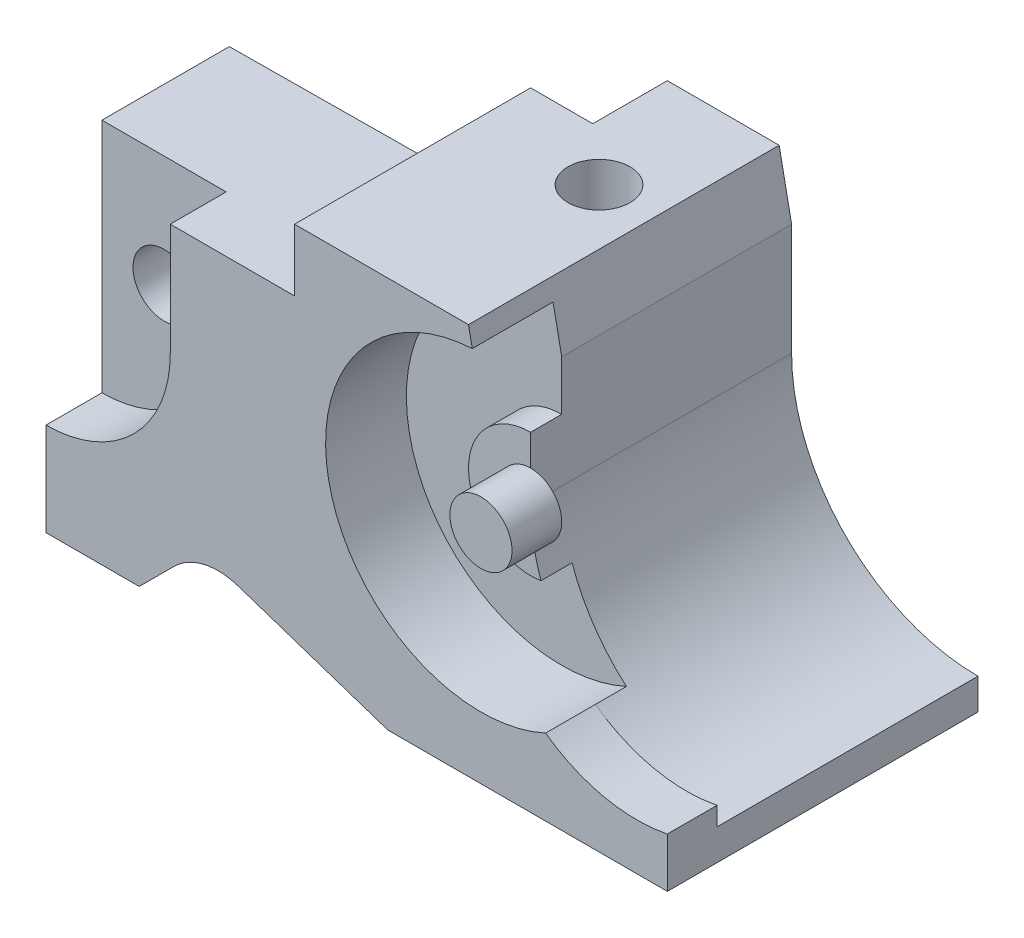
ISO-10303-21;
HEADER;
FILE_DESCRIPTION(('STEP AP214'),'2;1');
FILE_NAME('part.step','',(''),(''),'','','');
FILE_SCHEMA(('AUTOMOTIVE_DESIGN { 1 0 10303 214 1 1 1 1 }'));
ENDSEC;
DATA;
#1=APPLICATION_CONTEXT('core data for automotive mechanical design processes');
#2=APPLICATION_PROTOCOL_DEFINITION('international standard','automotive_design',2000,#1);
#3=PRODUCT_CONTEXT('',#1,'mechanical');
#4=PRODUCT('Part','Part','',(#3));
#5=PRODUCT_RELATED_PRODUCT_CATEGORY('part','',(#4));
#6=PRODUCT_DEFINITION_FORMATION('','',#4);
#7=PRODUCT_DEFINITION_CONTEXT('part definition',#1,'design');
#8=PRODUCT_DEFINITION('design','',#6,#7);
#9=PRODUCT_DEFINITION_SHAPE('','',#8);
#10=(LENGTH_UNIT() NAMED_UNIT(*) SI_UNIT(.MILLI.,.METRE.));
#11=(NAMED_UNIT(*) PLANE_ANGLE_UNIT() SI_UNIT($,.RADIAN.));
#12=(NAMED_UNIT(*) SI_UNIT($,.STERADIAN.) SOLID_ANGLE_UNIT());
#13=UNCERTAINTY_MEASURE_WITH_UNIT(LENGTH_MEASURE(1.E-05),#10,'distance_accuracy_value','');
#14=(GEOMETRIC_REPRESENTATION_CONTEXT(3) GLOBAL_UNCERTAINTY_ASSIGNED_CONTEXT((#13)) GLOBAL_UNIT_ASSIGNED_CONTEXT((#10,
#11,#12)) REPRESENTATION_CONTEXT('',''));
#15=CARTESIAN_POINT('',(0.,0.,0.));
#16=DIRECTION('',(0.,0.,1.));
#17=DIRECTION('',(1.,0.,0.));
#18=AXIS2_PLACEMENT_3D('',#15,#16,#17);
#19=CARTESIAN_POINT('',(0.,0.,50.));
#20=DIRECTION('',(0.,1.,0.));
#21=DIRECTION('',(0.,0.,1.));
#22=AXIS2_PLACEMENT_3D('',#19,#20,#21);
#23=PLANE('',#22);
#24=DIRECTION('',(-0.999964092712605,0.,0.00847427197214061));
#25=VECTOR('',#24,1.);
#26=CARTESIAN_POINT('',(0.173716337522439,0.,20.4985278276481));
#27=LINE('',#26,#25);
#28=CARTESIAN_POINT('',(15.,0.,20.3728813559322));
#29=VERTEX_POINT('',#28);
#30=CARTESIAN_POINT('',(0.,0.,20.5));
#31=VERTEX_POINT('',#30);
#32=EDGE_CURVE('E213',#29,#31,#27,.T.);
#33=ORIENTED_EDGE('',*,*,#32,.F.);
#34=DIRECTION('',(0.,0.,1.));
#35=VECTOR('',#34,1.);
#36=CARTESIAN_POINT('',(15.,0.,0.));
#37=LINE('',#36,#35);
#38=CARTESIAN_POINT('',(15.,0.,50.));
#39=VERTEX_POINT('',#38);
#40=EDGE_CURVE('E352',#29,#39,#37,.T.);
#41=ORIENTED_EDGE('',*,*,#40,.T.);
#42=DIRECTION('',(1.,0.,0.));
#43=VECTOR('',#42,1.);
#44=CARTESIAN_POINT('',(0.,0.,50.));
#45=LINE('',#44,#43);
#46=CARTESIAN_POINT('',(0.,0.,50.));
#47=VERTEX_POINT('',#46);
#48=EDGE_CURVE('E237',#47,#39,#45,.T.);
#49=ORIENTED_EDGE('',*,*,#48,.F.);
#50=DIRECTION('',(0.,0.,-1.));
#51=VECTOR('',#50,1.);
#52=CARTESIAN_POINT('',(0.,0.,50.));
#53=LINE('',#52,#51);
#54=EDGE_CURVE('E229',#47,#31,#53,.T.);
#55=ORIENTED_EDGE('',*,*,#54,.T.);
#56=EDGE_LOOP('',(#33,#41,#49,#55));
#57=FACE_BOUND('',#56,.T.);
#58=ADVANCED_FACE('F41',(#57),#23,.F.);
#59=CARTESIAN_POINT('',(0.,63.,50.));
#60=DIRECTION('',(0.,-1.,0.));
#61=DIRECTION('',(0.,0.,-1.));
#62=AXIS2_PLACEMENT_3D('',#59,#60,#61);
#63=PLANE('',#62);
#64=CARTESIAN_POINT('',(59.,63.,20.));
#65=DIRECTION('',(0.,1.,0.));
#66=DIRECTION('',(0.,0.,1.));
#67=AXIS2_PLACEMENT_3D('',#64,#65,#66);
#68=CIRCLE('',#67,5.);
#69=CARTESIAN_POINT('',(59.,63.,25.));
#70=VERTEX_POINT('',#69);
#71=EDGE_CURVE('E304',#70,#70,#68,.T.);
#72=ORIENTED_EDGE('',*,*,#71,.F.);
#73=EDGE_LOOP('',(#72));
#74=FACE_BOUND('',#73,.T.);
#75=DIRECTION('',(1.,0.,0.));
#76=VECTOR('',#75,1.);
#77=CARTESIAN_POINT('',(0.,63.,12.));
#78=LINE('',#77,#76);
#79=CARTESIAN_POINT('',(40.,63.,12.));
#80=VERTEX_POINT('',#79);
#81=CARTESIAN_POINT('',(50.,63.,12.));
#82=VERTEX_POINT('',#81);
#83=EDGE_CURVE('E303',#80,#82,#78,.T.);
#84=ORIENTED_EDGE('',*,*,#83,.F.);
#85=DIRECTION('',(0.,0.,-1.));
#86=VECTOR('',#85,1.);
#87=CARTESIAN_POINT('',(40.,63.,50.));
#88=LINE('',#87,#86);
#89=CARTESIAN_POINT('',(40.,63.,50.));
#90=VERTEX_POINT('',#89);
#91=EDGE_CURVE('E252',#90,#80,#88,.T.);
#92=ORIENTED_EDGE('',*,*,#91,.F.);
#93=DIRECTION('',(-1.,0.,0.));
#94=VECTOR('',#93,1.);
#95=CARTESIAN_POINT('',(0.,63.,50.));
#96=LINE('',#95,#94);
#97=CARTESIAN_POINT('',(68.,63.,50.));
#98=VERTEX_POINT('',#97);
#99=EDGE_CURVE('E423',#98,#90,#96,.T.);
#100=ORIENTED_EDGE('',*,*,#99,.F.);
#101=DIRECTION('',(0.,0.,-1.));
#102=VECTOR('',#101,1.);
#103=CARTESIAN_POINT('',(68.,63.,50.));
#104=LINE('',#103,#102);
#105=CARTESIAN_POINT('',(68.,63.,0.));
#106=VERTEX_POINT('',#105);
#107=EDGE_CURVE('E254',#98,#106,#104,.T.);
#108=ORIENTED_EDGE('',*,*,#107,.T.);
#109=DIRECTION('',(-1.,0.,0.));
#110=VECTOR('',#109,1.);
#111=CARTESIAN_POINT('',(0.,63.,0.));
#112=LINE('',#111,#110);
#113=CARTESIAN_POINT('',(50.,63.,0.));
#114=VERTEX_POINT('',#113);
#115=EDGE_CURVE('E445',#106,#114,#112,.T.);
#116=ORIENTED_EDGE('',*,*,#115,.T.);
#117=DIRECTION('',(0.,0.,-1.));
#118=VECTOR('',#117,1.);
#119=CARTESIAN_POINT('',(50.,63.,50.));
#120=LINE('',#119,#118);
#121=EDGE_CURVE('E301',#82,#114,#120,.T.);
#122=ORIENTED_EDGE('',*,*,#121,.F.);
#123=EDGE_LOOP('',(#84,#92,#100,#108,#116,#122));
#124=FACE_BOUND('',#123,.T.);
#125=ADVANCED_FACE('F494',(#74,#124),#63,.F.);
#126=CARTESIAN_POINT('',(40.,0.,50.));
#127=DIRECTION('',(1.,0.,0.));
#128=DIRECTION('',(0.,0.,-1.));
#129=AXIS2_PLACEMENT_3D('',#126,#127,#128);
#130=PLANE('',#129);
#131=ORIENTED_EDGE('',*,*,#91,.T.);
#132=DIRECTION('',(0.,1.,0.));
#133=VECTOR('',#132,1.);
#134=CARTESIAN_POINT('',(40.,0.,12.));
#135=LINE('',#134,#133);
#136=CARTESIAN_POINT('',(40.,5.,12.));
#137=VERTEX_POINT('',#136);
#138=EDGE_CURVE('E269',#137,#80,#135,.T.);
#139=ORIENTED_EDGE('',*,*,#138,.F.);
#140=DIRECTION('',(0.,0.,1.));
#141=VECTOR('',#140,1.);
#142=CARTESIAN_POINT('',(40.,5.,0.));
#143=LINE('',#142,#141);
#144=CARTESIAN_POINT('',(40.,4.99999999999999,20.1610169491525));
#145=VERTEX_POINT('',#144);
#146=EDGE_CURVE('E11',#137,#145,#143,.T.);
#147=ORIENTED_EDGE('',*,*,#146,.T.);
#148=DIRECTION('',(0.,1.,0.));
#149=VECTOR('',#148,1.);
#150=CARTESIAN_POINT('',(40.,0.,20.1610169491525));
#151=LINE('',#150,#149);
#152=CARTESIAN_POINT('',(40.,53.,20.1610169491525));
#153=VERTEX_POINT('',#152);
#154=EDGE_CURVE('E232',#145,#153,#151,.T.);
#155=ORIENTED_EDGE('',*,*,#154,.T.);
#156=DIRECTION('',(0.,0.,-1.));
#157=VECTOR('',#156,1.);
#158=CARTESIAN_POINT('',(40.,53.,50.));
#159=LINE('',#158,#157);
#160=CARTESIAN_POINT('',(40.,53.,50.));
#161=VERTEX_POINT('',#160);
#162=EDGE_CURVE('E245',#161,#153,#159,.T.);
#163=ORIENTED_EDGE('',*,*,#162,.F.);
#164=DIRECTION('',(0.,-1.,0.));
#165=VECTOR('',#164,1.);
#166=CARTESIAN_POINT('',(40.,0.,50.));
#167=LINE('',#166,#165);
#168=EDGE_CURVE('E425',#90,#161,#167,.T.);
#169=ORIENTED_EDGE('',*,*,#168,.F.);
#170=EDGE_LOOP('',(#131,#139,#147,#155,#163,#169));
#171=FACE_BOUND('',#170,.T.);
#172=ADVANCED_FACE('F286',(#171),#130,.F.);
#173=CARTESIAN_POINT('',(0.,53.,50.));
#174=DIRECTION('',(0.,-1.,0.));
#175=DIRECTION('',(0.,0.,-1.));
#176=AXIS2_PLACEMENT_3D('',#173,#174,#175);
#177=PLANE('',#176);
#178=DIRECTION('',(0.999964092712605,0.,-0.00847427197214061));
#179=VECTOR('',#178,1.);
#180=CARTESIAN_POINT('',(-0.249982046678632,53.,20.502118491921));
#181=LINE('',#180,#179);
#182=CARTESIAN_POINT('',(0.,53.,20.5));
#183=VERTEX_POINT('',#182);
#184=EDGE_CURVE('E287',#183,#153,#181,.T.);
#185=ORIENTED_EDGE('',*,*,#184,.F.);
#186=DIRECTION('',(0.,0.,-1.));
#187=VECTOR('',#186,1.);
#188=CARTESIAN_POINT('',(0.,53.,50.));
#189=LINE('',#188,#187);
#190=CARTESIAN_POINT('',(0.,53.,41.));
#191=VERTEX_POINT('',#190);
#192=EDGE_CURVE('E234',#191,#183,#189,.T.);
#193=ORIENTED_EDGE('',*,*,#192,.F.);
#194=DIRECTION('',(-1.,0.,0.));
#195=VECTOR('',#194,1.);
#196=CARTESIAN_POINT('',(0.,53.,41.));
#197=LINE('',#196,#195);
#198=CARTESIAN_POINT('',(20.,53.,41.));
#199=VERTEX_POINT('',#198);
#200=EDGE_CURVE('E325',#199,#191,#197,.T.);
#201=ORIENTED_EDGE('',*,*,#200,.F.);
#202=DIRECTION('',(0.,0.,1.));
#203=VECTOR('',#202,1.);
#204=CARTESIAN_POINT('',(20.,53.,41.));
#205=LINE('',#204,#203);
#206=CARTESIAN_POINT('',(20.,53.,50.));
#207=VERTEX_POINT('',#206);
#208=EDGE_CURVE('E328',#199,#207,#205,.T.);
#209=ORIENTED_EDGE('',*,*,#208,.T.);
#210=DIRECTION('',(-1.,0.,0.));
#211=VECTOR('',#210,1.);
#212=CARTESIAN_POINT('',(0.,53.,50.));
#213=LINE('',#212,#211);
#214=EDGE_CURVE('E428',#161,#207,#213,.T.);
#215=ORIENTED_EDGE('',*,*,#214,.F.);
#216=ORIENTED_EDGE('',*,*,#162,.T.);
#217=EDGE_LOOP('',(#185,#193,#201,#209,#215,#216));
#218=FACE_BOUND('',#217,.T.);
#219=ADVANCED_FACE('F538',(#218),#177,.F.);
#220=CARTESIAN_POINT('',(0.,0.,50.));
#221=DIRECTION('',(1.,0.,0.));
#222=DIRECTION('',(0.,0.,-1.));
#223=AXIS2_PLACEMENT_3D('',#220,#221,#222);
#224=PLANE('',#223);
#225=DIRECTION('',(0.,1.,0.));
#226=VECTOR('',#225,1.);
#227=CARTESIAN_POINT('',(0.,0.,20.5));
#228=LINE('',#227,#226);
#229=EDGE_CURVE('E217',#31,#183,#228,.T.);
#230=ORIENTED_EDGE('',*,*,#229,.F.);
#231=ORIENTED_EDGE('',*,*,#54,.F.);
#232=DIRECTION('',(0.,-1.,0.));
#233=VECTOR('',#232,1.);
#234=CARTESIAN_POINT('',(0.,0.,50.));
#235=LINE('',#234,#233);
#236=CARTESIAN_POINT('',(0.,15.,50.));
#237=VERTEX_POINT('',#236);
#238=EDGE_CURVE('E429',#237,#47,#235,.T.);
#239=ORIENTED_EDGE('',*,*,#238,.F.);
#240=DIRECTION('',(0.,0.,1.));
#241=VECTOR('',#240,1.);
#242=CARTESIAN_POINT('',(0.,15.,41.));
#243=LINE('',#242,#241);
#244=CARTESIAN_POINT('',(0.,15.,41.));
#245=VERTEX_POINT('',#244);
#246=EDGE_CURVE('E322',#245,#237,#243,.T.);
#247=ORIENTED_EDGE('',*,*,#246,.F.);
#248=DIRECTION('',(0.,-1.,0.));
#249=VECTOR('',#248,1.);
#250=CARTESIAN_POINT('',(0.,0.,41.));
#251=LINE('',#250,#249);
#252=EDGE_CURVE('E312',#191,#245,#251,.T.);
#253=ORIENTED_EDGE('',*,*,#252,.F.);
#254=ORIENTED_EDGE('',*,*,#192,.T.);
#255=EDGE_LOOP('',(#230,#231,#239,#247,#253,#254));
#256=FACE_BOUND('',#255,.T.);
#257=ADVANCED_FACE('F226',(#256),#224,.F.);
#258=CARTESIAN_POINT('',(0.,0.,0.));
#259=DIRECTION('',(0.,0.,1.));
#260=DIRECTION('',(1.,0.,0.));
#261=AXIS2_PLACEMENT_3D('',#258,#259,#260);
#262=PLANE('',#261);
#263=DIRECTION('',(0.,1.,0.));
#264=VECTOR('',#263,1.);
#265=CARTESIAN_POINT('',(50.,0.,0.));
#266=LINE('',#265,#264);
#267=CARTESIAN_POINT('',(50.,1.66666666666666,0.));
#268=VERTEX_POINT('',#267);
#269=EDGE_CURVE('E236',#268,#114,#266,.T.);
#270=ORIENTED_EDGE('',*,*,#269,.T.);
#271=ORIENTED_EDGE('',*,*,#115,.F.);
#272=DIRECTION('',(-0.196116135138184,0.98058067569092,0.));
#273=VECTOR('',#272,1.);
#274=CARTESIAN_POINT('',(77.5,15.5,0.));
#275=LINE('',#274,#273);
#276=CARTESIAN_POINT('',(70.,53.,0.));
#277=VERTEX_POINT('',#276);
#278=EDGE_CURVE('E439',#277,#106,#275,.T.);
#279=ORIENTED_EDGE('',*,*,#278,.F.);
#280=DIRECTION('',(0.,1.,0.));
#281=VECTOR('',#280,1.);
#282=CARTESIAN_POINT('',(70.,0.,0.));
#283=LINE('',#282,#281);
#284=CARTESIAN_POINT('',(70.,35.,0.));
#285=VERTEX_POINT('',#284);
#286=EDGE_CURVE('E440',#285,#277,#283,.T.);
#287=ORIENTED_EDGE('',*,*,#286,.F.);
#288=CARTESIAN_POINT('',(100.,35.,0.));
#289=DIRECTION('',(0.,0.,1.));
#290=DIRECTION('',(1.,0.,0.));
#291=AXIS2_PLACEMENT_3D('',#288,#289,#290);
#292=CIRCLE('',#291,30.);
#293=CARTESIAN_POINT('',(100.,5.00000000000002,0.));
#294=VERTEX_POINT('',#293);
#295=EDGE_CURVE('E411',#285,#294,#292,.T.);
#296=ORIENTED_EDGE('',*,*,#295,.T.);
#297=DIRECTION('',(0.,1.,0.));
#298=VECTOR('',#297,1.);
#299=CARTESIAN_POINT('',(100.,0.,0.));
#300=LINE('',#299,#298);
#301=CARTESIAN_POINT('',(100.,0.,0.));
#302=VERTEX_POINT('',#301);
#303=EDGE_CURVE('E422',#302,#294,#300,.T.);
#304=ORIENTED_EDGE('',*,*,#303,.F.);
#305=DIRECTION('',(1.,0.,0.));
#306=VECTOR('',#305,1.);
#307=CARTESIAN_POINT('',(0.,0.,0.));
#308=LINE('',#307,#306);
#309=CARTESIAN_POINT('',(55.,0.,0.));
#310=VERTEX_POINT('',#309);
#311=EDGE_CURVE('E444',#310,#302,#308,.T.);
#312=ORIENTED_EDGE('',*,*,#311,.F.);
#313=DIRECTION('',(-0.948683298050514,0.316227766016838,0.));
#314=VECTOR('',#313,1.);
#315=CARTESIAN_POINT('',(5.5,16.5,0.));
#316=LINE('',#315,#314);
#317=EDGE_CURVE('E337',#310,#268,#316,.T.);
#318=ORIENTED_EDGE('',*,*,#317,.T.);
#319=EDGE_LOOP('',(#270,#271,#279,#287,#296,#304,#312,#318));
#320=FACE_BOUND('',#319,.T.);
#321=ADVANCED_FACE('F465',(#320),#262,.F.);
#322=CARTESIAN_POINT('',(27.7009075673773,-1.44122805635369,0.));
#323=DIRECTION('',(0.,0.,1.));
#324=DIRECTION('',(1.,0.,0.));
#325=AXIS2_PLACEMENT_3D('',#322,#323,#324);
#326=CYLINDRICAL_SURFACE('',#325,9.99999999999999);
#327=DIRECTION('',(0.,0.,1.));
#328=VECTOR('',#327,1.);
#329=CARTESIAN_POINT('',(20.6298397555118,5.62983975551179,0.));
#330=LINE('',#329,#328);
#331=CARTESIAN_POINT('',(20.6298397555118,5.62983975551179,20.3251708495296));
#332=VERTEX_POINT('',#331);
#333=CARTESIAN_POINT('',(20.6298397555118,5.62983975551179,50.));
#334=VERTEX_POINT('',#333);
#335=EDGE_CURVE('E339',#332,#334,#330,.T.);
#336=ORIENTED_EDGE('',*,*,#335,.F.);
#337=CARTESIAN_POINT('',(27.7009075673773,-1.44122805635369,20.2652465460392));
#338=DIRECTION('',(-0.00847427197214061,0.,-0.999964092712605));
#339=DIRECTION('',(-0.999964092712605,0.,0.00847427197214061));
#340=AXIS2_PLACEMENT_3D('',#337,#338,#339);
#341=ELLIPSE('',#340,10.0003590857677,9.99999999999999);
#342=CARTESIAN_POINT('',(30.8631852275457,8.04560492415144,20.2384475828174));
#343=VERTEX_POINT('',#342);
#344=EDGE_CURVE('E57',#332,#343,#341,.T.);
#345=ORIENTED_EDGE('',*,*,#344,.T.);
#346=DIRECTION('',(0.,0.,1.));
#347=VECTOR('',#346,1.);
#348=CARTESIAN_POINT('',(30.8631852275457,8.04560492415144,0.));
#349=LINE('',#348,#347);
#350=CARTESIAN_POINT('',(30.8631852275457,8.04560492415144,50.));
#351=VERTEX_POINT('',#350);
#352=EDGE_CURVE('E349',#343,#351,#349,.T.);
#353=ORIENTED_EDGE('',*,*,#352,.T.);
#354=CARTESIAN_POINT('',(27.7009075673773,-1.44122805635369,50.));
#355=DIRECTION('',(0.,0.,1.));
#356=DIRECTION('',(1.,0.,0.));
#357=AXIS2_PLACEMENT_3D('',#354,#355,#356);
#358=CIRCLE('',#357,9.99999999999999);
#359=EDGE_CURVE('E335',#334,#351,#358,.F.);
#360=ORIENTED_EDGE('',*,*,#359,.F.);
#361=EDGE_LOOP('',(#336,#345,#353,#360));
#362=FACE_BOUND('',#361,.T.);
#363=ADVANCED_FACE('F530',(#362),#326,.F.);
#364=CARTESIAN_POINT('',(5.5,16.5,0.));
#365=DIRECTION('',(0.316227766016838,0.948683298050514,0.));
#366=DIRECTION('',(-0.948683298050514,0.316227766016838,0.));
#367=AXIS2_PLACEMENT_3D('',#364,#365,#366);
#368=PLANE('',#367);
#369=DIRECTION('',(-0.94865263970594,0.316217546568647,0.00803942915005023));
#370=VECTOR('',#369,1.);
#371=CARTESIAN_POINT('',(5.65599034822512,16.4480032172583,20.4520678784049));
#372=LINE('',#371,#370);
#373=EDGE_CURVE('E283',#145,#343,#372,.T.);
#374=ORIENTED_EDGE('',*,*,#373,.F.);
#375=ORIENTED_EDGE('',*,*,#146,.F.);
#376=DIRECTION('',(-0.948683298050514,0.316227766016838,0.));
#377=VECTOR('',#376,1.);
#378=CARTESIAN_POINT('',(5.5,16.5,12.));
#379=LINE('',#378,#377);
#380=CARTESIAN_POINT('',(50.,1.66666666666666,12.));
#381=VERTEX_POINT('',#380);
#382=EDGE_CURVE('E47',#381,#137,#379,.T.);
#383=ORIENTED_EDGE('',*,*,#382,.F.);
#384=DIRECTION('',(0.,0.,1.));
#385=VECTOR('',#384,1.);
#386=CARTESIAN_POINT('',(50.,1.66666666666666,0.));
#387=LINE('',#386,#385);
#388=EDGE_CURVE('E265',#268,#381,#387,.T.);
#389=ORIENTED_EDGE('',*,*,#388,.F.);
#390=ORIENTED_EDGE('',*,*,#317,.F.);
#391=DIRECTION('',(0.,0.,1.));
#392=VECTOR('',#391,1.);
#393=CARTESIAN_POINT('',(55.,0.,0.));
#394=LINE('',#393,#392);
#395=CARTESIAN_POINT('',(55.,0.,17.));
#396=VERTEX_POINT('',#395);
#397=EDGE_CURVE('E353',#310,#396,#394,.T.);
#398=ORIENTED_EDGE('',*,*,#397,.T.);
#399=CARTESIAN_POINT('',(59.,-1.33333333333334,20.));
#400=DIRECTION('',(0.316227766016838,0.948683298050514,0.));
#401=DIRECTION('',(-0.948683298050514,0.316227766016838,0.));
#402=AXIS2_PLACEMENT_3D('',#399,#400,#401);
#403=ELLIPSE('',#402,5.2704627669473,5.);
#404=CARTESIAN_POINT('',(55.,0.,23.));
#405=VERTEX_POINT('',#404);
#406=EDGE_CURVE('E264',#396,#405,#403,.T.);
#407=ORIENTED_EDGE('',*,*,#406,.T.);
#408=CARTESIAN_POINT('',(55.,0.,50.));
#409=VERTEX_POINT('',#408);
#410=EDGE_CURVE('E354',#405,#409,#394,.T.);
#411=ORIENTED_EDGE('',*,*,#410,.T.);
#412=DIRECTION('',(-0.948683298050514,0.316227766016838,0.));
#413=VECTOR('',#412,1.);
#414=CARTESIAN_POINT('',(5.5,16.5,50.));
#415=LINE('',#414,#413);
#416=EDGE_CURVE('E338',#409,#351,#415,.T.);
#417=ORIENTED_EDGE('',*,*,#416,.T.);
#418=ORIENTED_EDGE('',*,*,#352,.F.);
#419=EDGE_LOOP('',(#374,#375,#383,#389,#390,#398,#407,#411,#417,#418));
#420=FACE_BOUND('',#419,.T.);
#421=ADVANCED_FACE('F282',(#420),#368,.F.);
#422=CARTESIAN_POINT('',(7.49999999999995,-7.5,0.));
#423=DIRECTION('',(0.707106781186545,-0.70710678118655,0.));
#424=DIRECTION('',(0.70710678118655,0.707106781186545,0.));
#425=AXIS2_PLACEMENT_3D('',#422,#423,#424);
#426=PLANE('',#425);
#427=ORIENTED_EDGE('',*,*,#40,.F.);
#428=DIRECTION('',(0.707094085701452,0.707094085701447,-0.00599232276018172));
#429=VECTOR('',#428,1.);
#430=CARTESIAN_POINT('',(7.58659197816793,-7.41340802183202,20.4357068476426));
#431=LINE('',#430,#429);
#432=EDGE_CURVE('E218',#29,#332,#431,.T.);
#433=ORIENTED_EDGE('',*,*,#432,.T.);
#434=ORIENTED_EDGE('',*,*,#335,.T.);
#435=DIRECTION('',(0.70710678118655,0.707106781186545,0.));
#436=VECTOR('',#435,1.);
#437=CARTESIAN_POINT('',(7.49999999999995,-7.5,50.));
#438=LINE('',#437,#436);
#439=EDGE_CURVE('E345',#39,#334,#438,.T.);
#440=ORIENTED_EDGE('',*,*,#439,.F.);
#441=EDGE_LOOP('',(#427,#433,#434,#440));
#442=FACE_BOUND('',#441,.T.);
#443=ADVANCED_FACE('F529',(#442),#426,.T.);
#444=CARTESIAN_POINT('',(10.,35.,0.));
#445=DIRECTION('',(0.,0.,1.));
#446=DIRECTION('',(1.,0.,0.));
#447=AXIS2_PLACEMENT_3D('',#444,#445,#446);
#448=CYLINDRICAL_SURFACE('',#447,5.00000000000001);
#449=CARTESIAN_POINT('',(10.,35.,41.));
#450=DIRECTION('',(0.,0.,1.));
#451=DIRECTION('',(1.,0.,0.));
#452=AXIS2_PLACEMENT_3D('',#449,#450,#451);
#453=CIRCLE('',#452,5.00000000000001);
#454=CARTESIAN_POINT('',(15.,35.,41.));
#455=VERTEX_POINT('',#454);
#456=EDGE_CURVE('E310',#455,#455,#453,.T.);
#457=ORIENTED_EDGE('',*,*,#456,.T.);
#458=EDGE_LOOP('',(#457));
#459=FACE_BOUND('',#458,.T.);
#460=CARTESIAN_POINT('',(10.,35.,20.4152542372881));
#461=DIRECTION('',(-0.00847427197214061,0.,-0.999964092712605));
#462=DIRECTION('',(-0.999964092712605,0.,0.00847427197214061));
#463=AXIS2_PLACEMENT_3D('',#460,#461,#462);
#464=ELLIPSE('',#463,5.00017954288388,5.00000000000001);
#465=CARTESIAN_POINT('',(5.,35.,20.4576271186441));
#466=VERTEX_POINT('',#465);
#467=EDGE_CURVE('E268',#466,#466,#464,.F.);
#468=ORIENTED_EDGE('',*,*,#467,.F.);
#469=EDGE_LOOP('',(#468));
#470=FACE_BOUND('',#469,.T.);
#471=ADVANCED_FACE('F575',(#459,#470),#448,.F.);
#472=CARTESIAN_POINT('',(100.,35.,50.));
#473=DIRECTION('',(0.,0.,-1.));
#474=DIRECTION('',(-1.,0.,0.));
#475=AXIS2_PLACEMENT_3D('',#472,#473,#474);
#476=CYLINDRICAL_SURFACE('',#475,30.);
#477=DIRECTION('',(0.,0.,1.));
#478=VECTOR('',#477,1.);
#479=CARTESIAN_POINT('',(80.4166666666667,12.2735164278423,37.));
#480=LINE('',#479,#478);
#481=CARTESIAN_POINT('',(80.4166666666667,12.2735164278423,37.));
#482=VERTEX_POINT('',#481);
#483=CARTESIAN_POINT('',(80.4166666666667,12.2735164278423,42.));
#484=VERTEX_POINT('',#483);
#485=EDGE_CURVE('E412',#482,#484,#480,.T.);
#486=ORIENTED_EDGE('',*,*,#485,.T.);
#487=CARTESIAN_POINT('',(100.,35.,42.));
#488=DIRECTION('',(0.,0.,1.));
#489=DIRECTION('',(1.,0.,0.));
#490=AXIS2_PLACEMENT_3D('',#487,#488,#489);
#491=CIRCLE('',#490,30.);
#492=CARTESIAN_POINT('',(100.,5.00000000000002,42.));
#493=VERTEX_POINT('',#492);
#494=EDGE_CURVE('E367',#484,#493,#491,.T.);
#495=ORIENTED_EDGE('',*,*,#494,.T.);
#496=DIRECTION('',(0.,0.,-1.));
#497=VECTOR('',#496,1.);
#498=CARTESIAN_POINT('',(100.,5.00000000000002,50.));
#499=LINE('',#498,#497);
#500=EDGE_CURVE('E244',#493,#294,#499,.T.);
#501=ORIENTED_EDGE('',*,*,#500,.T.);
#502=ORIENTED_EDGE('',*,*,#295,.F.);
#503=DIRECTION('',(0.,0.,-1.));
#504=VECTOR('',#503,1.);
#505=CARTESIAN_POINT('',(70.,35.,50.));
#506=LINE('',#505,#504);
#507=CARTESIAN_POINT('',(70.,35.,42.));
#508=VERTEX_POINT('',#507);
#509=EDGE_CURVE('E260',#508,#285,#506,.T.);
#510=ORIENTED_EDGE('',*,*,#509,.F.);
#511=CARTESIAN_POINT('',(100.,35.,42.));
#512=DIRECTION('',(0.,0.,1.));
#513=DIRECTION('',(1.,0.,0.));
#514=AXIS2_PLACEMENT_3D('',#511,#512,#513);
#515=CIRCLE('',#514,30.);
#516=CARTESIAN_POINT('',(70.4166666666667,30.0173913570411,42.));
#517=VERTEX_POINT('',#516);
#518=EDGE_CURVE('E377',#508,#517,#515,.T.);
#519=ORIENTED_EDGE('',*,*,#518,.T.);
#520=CARTESIAN_POINT('',(100.,35.,42.));
#521=DIRECTION('',(0.,0.,1.));
#522=DIRECTION('',(1.,0.,0.));
#523=AXIS2_PLACEMENT_3D('',#520,#521,#522);
#524=CIRCLE('',#523,30.);
#525=CARTESIAN_POINT('',(71.6666666666667,25.1398670281673,42.));
#526=VERTEX_POINT('',#525);
#527=EDGE_CURVE('E388',#517,#526,#524,.T.);
#528=ORIENTED_EDGE('',*,*,#527,.T.);
#529=DIRECTION('',(0.,0.,1.));
#530=VECTOR('',#529,1.);
#531=CARTESIAN_POINT('',(71.6666666666667,25.1398670281673,37.));
#532=LINE('',#531,#530);
#533=CARTESIAN_POINT('',(71.6666666666667,25.1398670281673,37.));
#534=VERTEX_POINT('',#533);
#535=EDGE_CURVE('E410',#534,#526,#532,.T.);
#536=ORIENTED_EDGE('',*,*,#535,.F.);
#537=CARTESIAN_POINT('',(100.,35.,37.));
#538=DIRECTION('',(0.,0.,1.));
#539=DIRECTION('',(1.,0.,0.));
#540=AXIS2_PLACEMENT_3D('',#537,#538,#539);
#541=CIRCLE('',#540,30.);
#542=EDGE_CURVE('E401',#482,#534,#541,.F.);
#543=ORIENTED_EDGE('',*,*,#542,.F.);
#544=EDGE_LOOP('',(#486,#495,#501,#502,#510,#519,#528,#536,#543));
#545=FACE_BOUND('',#544,.T.);
#546=ADVANCED_FACE('F43',(#545),#476,.F.);
#547=CARTESIAN_POINT('',(70.,0.,50.));
#548=DIRECTION('',(-1.,0.,0.));
#549=DIRECTION('',(0.,0.,1.));
#550=AXIS2_PLACEMENT_3D('',#547,#548,#549);
#551=PLANE('',#550);
#552=DIRECTION('',(0.,1.,0.));
#553=VECTOR('',#552,1.);
#554=CARTESIAN_POINT('',(70.,0.,42.));
#555=LINE('',#554,#553);
#556=CARTESIAN_POINT('',(70.,40.,42.));
#557=VERTEX_POINT('',#556);
#558=EDGE_CURVE('E376',#508,#557,#555,.T.);
#559=ORIENTED_EDGE('',*,*,#558,.F.);
#560=ORIENTED_EDGE('',*,*,#509,.T.);
#561=ORIENTED_EDGE('',*,*,#286,.T.);
#562=DIRECTION('',(0.,0.,-1.));
#563=VECTOR('',#562,1.);
#564=CARTESIAN_POINT('',(70.,53.,50.));
#565=LINE('',#564,#563);
#566=CARTESIAN_POINT('',(70.,53.,37.));
#567=VERTEX_POINT('',#566);
#568=EDGE_CURVE('E259',#567,#277,#565,.T.);
#569=ORIENTED_EDGE('',*,*,#568,.F.);
#570=DIRECTION('',(0.,1.,0.));
#571=VECTOR('',#570,1.);
#572=CARTESIAN_POINT('',(70.,0.,37.));
#573=LINE('',#572,#571);
#574=CARTESIAN_POINT('',(70.,45.,37.));
#575=VERTEX_POINT('',#574);
#576=EDGE_CURVE('E395',#575,#567,#573,.T.);
#577=ORIENTED_EDGE('',*,*,#576,.F.);
#578=DIRECTION('',(0.,0.,1.));
#579=VECTOR('',#578,1.);
#580=CARTESIAN_POINT('',(70.,45.,37.));
#581=LINE('',#580,#579);
#582=CARTESIAN_POINT('',(70.,45.,42.));
#583=VERTEX_POINT('',#582);
#584=EDGE_CURVE('E409',#575,#583,#581,.T.);
#585=ORIENTED_EDGE('',*,*,#584,.T.);
#586=DIRECTION('',(0.,1.,0.));
#587=VECTOR('',#586,1.);
#588=CARTESIAN_POINT('',(70.,0.,42.));
#589=LINE('',#588,#587);
#590=EDGE_CURVE('E383',#557,#583,#589,.T.);
#591=ORIENTED_EDGE('',*,*,#590,.F.);
#592=EDGE_LOOP('',(#559,#560,#561,#569,#577,#585,#591));
#593=FACE_BOUND('',#592,.T.);
#594=ADVANCED_FACE('F466',(#593),#551,.F.);
#595=CARTESIAN_POINT('',(0.,0.,50.));
#596=DIRECTION('',(0.,0.,1.));
#597=DIRECTION('',(1.,0.,0.));
#598=AXIS2_PLACEMENT_3D('',#595,#596,#597);
#599=PLANE('',#598);
#600=CARTESIAN_POINT('',(70.,35.,50.));
#601=DIRECTION('',(0.,0.,1.));
#602=DIRECTION('',(1.,0.,0.));
#603=AXIS2_PLACEMENT_3D('',#600,#601,#602);
#604=CIRCLE('',#603,5.);
#605=CARTESIAN_POINT('',(75.,35.,50.));
#606=VERTEX_POINT('',#605);
#607=EDGE_CURVE('E382',#606,#606,#604,.T.);
#608=ORIENTED_EDGE('',*,*,#607,.T.);
#609=EDGE_LOOP('',(#608));
#610=FACE_BOUND('',#609,.T.);
#611=ADVANCED_FACE('F716',(#610),#599,.T.);
#612=CARTESIAN_POINT('',(70.,35.,37.));
#613=DIRECTION('',(0.,0.,1.));
#614=DIRECTION('',(1.,0.,0.));
#615=AXIS2_PLACEMENT_3D('',#612,#613,#614);
#616=CYLINDRICAL_SURFACE('',#615,9.99999999999999);
#617=ORIENTED_EDGE('',*,*,#535,.T.);
#618=CARTESIAN_POINT('',(70.,35.,42.));
#619=DIRECTION('',(0.,0.,1.));
#620=DIRECTION('',(1.,0.,0.));
#621=AXIS2_PLACEMENT_3D('',#618,#619,#620);
#622=CIRCLE('',#621,9.99999999999999);
#623=EDGE_CURVE('E257',#526,#583,#622,.F.);
#624=ORIENTED_EDGE('',*,*,#623,.T.);
#625=ORIENTED_EDGE('',*,*,#584,.F.);
#626=CARTESIAN_POINT('',(70.,35.,37.));
#627=DIRECTION('',(0.,0.,1.));
#628=DIRECTION('',(1.,0.,0.));
#629=AXIS2_PLACEMENT_3D('',#626,#627,#628);
#630=CIRCLE('',#629,9.99999999999999);
#631=EDGE_CURVE('E394',#575,#534,#630,.T.);
#632=ORIENTED_EDGE('',*,*,#631,.T.);
#633=EDGE_LOOP('',(#617,#624,#625,#632));
#634=FACE_BOUND('',#633,.T.);
#635=ADVANCED_FACE('F511',(#634),#616,.T.);
#636=CARTESIAN_POINT('',(77.5,15.5,50.));
#637=DIRECTION('',(-0.98058067569092,-0.196116135138184,0.));
#638=DIRECTION('',(0.196116135138184,-0.98058067569092,0.));
#639=AXIS2_PLACEMENT_3D('',#636,#637,#638);
#640=PLANE('',#639);
#641=DIRECTION('',(-0.196116135138184,0.98058067569092,0.));
#642=VECTOR('',#641,1.);
#643=CARTESIAN_POINT('',(77.5,15.5,50.));
#644=LINE('',#643,#642);
#645=CARTESIAN_POINT('',(68.6077593567962,59.9612032160193,50.));
#646=VERTEX_POINT('',#645);
#647=EDGE_CURVE('E419',#646,#98,#644,.T.);
#648=ORIENTED_EDGE('',*,*,#647,.F.);
#649=DIRECTION('',(0.,0.,1.));
#650=VECTOR('',#649,1.);
#651=CARTESIAN_POINT('',(68.6077593567961,59.9612032160193,37.));
#652=LINE('',#651,#650);
#653=CARTESIAN_POINT('',(68.6077593567961,59.9612032160193,37.));
#654=VERTEX_POINT('',#653);
#655=EDGE_CURVE('E415',#654,#646,#652,.T.);
#656=ORIENTED_EDGE('',*,*,#655,.F.);
#657=DIRECTION('',(-0.196116135138184,0.98058067569092,0.));
#658=VECTOR('',#657,1.);
#659=CARTESIAN_POINT('',(77.5,15.5,37.));
#660=LINE('',#659,#658);
#661=EDGE_CURVE('E400',#567,#654,#660,.T.);
#662=ORIENTED_EDGE('',*,*,#661,.F.);
#663=ORIENTED_EDGE('',*,*,#568,.T.);
#664=ORIENTED_EDGE('',*,*,#278,.T.);
#665=ORIENTED_EDGE('',*,*,#107,.F.);
#666=EDGE_LOOP('',(#648,#656,#662,#663,#664,#665));
#667=FACE_BOUND('',#666,.T.);
#668=ADVANCED_FACE('F506',(#667),#640,.F.);
#669=ORIENTED_EDGE('',*,*,#410,.F.);
#670=CARTESIAN_POINT('',(59.,0.,20.));
#671=DIRECTION('',(0.,1.,0.));
#672=DIRECTION('',(0.,0.,1.));
#673=AXIS2_PLACEMENT_3D('',#670,#671,#672);
#674=CIRCLE('',#673,5.);
#675=EDGE_CURVE('E65',#405,#396,#674,.T.);
#676=ORIENTED_EDGE('',*,*,#675,.T.);
#677=ORIENTED_EDGE('',*,*,#397,.F.);
#678=ORIENTED_EDGE('',*,*,#311,.T.);
#679=DIRECTION('',(0.,0.,-1.));
#680=VECTOR('',#679,1.);
#681=CARTESIAN_POINT('',(100.,0.,50.));
#682=LINE('',#681,#680);
#683=CARTESIAN_POINT('',(100.,0.,50.));
#684=VERTEX_POINT('',#683);
#685=EDGE_CURVE('E239',#684,#302,#682,.T.);
#686=ORIENTED_EDGE('',*,*,#685,.F.);
#687=EDGE_CURVE('E431',#409,#684,#45,.T.);
#688=ORIENTED_EDGE('',*,*,#687,.F.);
#689=EDGE_LOOP('',(#669,#676,#677,#678,#686,#688));
#690=FACE_BOUND('',#689,.T.);
#691=ADVANCED_FACE('F496',(#690),#23,.F.);
#692=CARTESIAN_POINT('',(100.,0.,50.));
#693=DIRECTION('',(-1.,0.,0.));
#694=DIRECTION('',(0.,0.,1.));
#695=AXIS2_PLACEMENT_3D('',#692,#693,#694);
#696=PLANE('',#695);
#697=ORIENTED_EDGE('',*,*,#685,.T.);
#698=ORIENTED_EDGE('',*,*,#303,.T.);
#699=ORIENTED_EDGE('',*,*,#500,.F.);
#700=DIRECTION('',(0.,1.,0.));
#701=VECTOR('',#700,1.);
#702=CARTESIAN_POINT('',(100.,0.,42.));
#703=LINE('',#702,#701);
#704=CARTESIAN_POINT('',(100.,8.,42.));
#705=VERTEX_POINT('',#704);
#706=EDGE_CURVE('E363',#493,#705,#703,.T.);
#707=ORIENTED_EDGE('',*,*,#706,.T.);
#708=DIRECTION('',(0.,0.,1.));
#709=VECTOR('',#708,1.);
#710=CARTESIAN_POINT('',(100.,8.,42.));
#711=LINE('',#710,#709);
#712=CARTESIAN_POINT('',(100.,8.,50.));
#713=VERTEX_POINT('',#712);
#714=EDGE_CURVE('E366',#705,#713,#711,.T.);
#715=ORIENTED_EDGE('',*,*,#714,.T.);
#716=DIRECTION('',(0.,1.,0.));
#717=VECTOR('',#716,1.);
#718=CARTESIAN_POINT('',(100.,0.,50.));
#719=LINE('',#718,#717);
#720=EDGE_CURVE('E433',#684,#713,#719,.T.);
#721=ORIENTED_EDGE('',*,*,#720,.F.);
#722=EDGE_LOOP('',(#697,#698,#699,#707,#715,#721));
#723=FACE_BOUND('',#722,.T.);
#724=ADVANCED_FACE('F456',(#723),#696,.F.);
#725=DIRECTION('',(0.,1.,0.));
#726=VECTOR('',#725,1.);
#727=CARTESIAN_POINT('',(20.,0.,50.));
#728=LINE('',#727,#726);
#729=CARTESIAN_POINT('',(20.,35.,50.));
#730=VERTEX_POINT('',#729);
#731=EDGE_CURVE('E320',#730,#207,#728,.T.);
#732=ORIENTED_EDGE('',*,*,#731,.F.);
#733=CARTESIAN_POINT('',(0.,35.,50.));
#734=DIRECTION('',(0.,0.,1.));
#735=DIRECTION('',(1.,0.,0.));
#736=AXIS2_PLACEMENT_3D('',#733,#734,#735);
#737=CIRCLE('',#736,20.);
#738=EDGE_CURVE('E315',#237,#730,#737,.T.);
#739=ORIENTED_EDGE('',*,*,#738,.F.);
#740=ORIENTED_EDGE('',*,*,#238,.T.);
#741=ORIENTED_EDGE('',*,*,#48,.T.);
#742=ORIENTED_EDGE('',*,*,#439,.T.);
#743=ORIENTED_EDGE('',*,*,#359,.T.);
#744=ORIENTED_EDGE('',*,*,#416,.F.);
#745=ORIENTED_EDGE('',*,*,#687,.T.);
#746=ORIENTED_EDGE('',*,*,#720,.T.);
#747=CARTESIAN_POINT('',(95.091406687724,32.5133782187335,50.));
#748=DIRECTION('',(0.,0.,-1.));
#749=DIRECTION('',(1.,0.,0.));
#750=AXIS2_PLACEMENT_3D('',#747,#748,#749);
#751=CIRCLE('',#750,25.);
#752=CARTESIAN_POINT('',(80.4166666666667,12.2735164278423,50.));
#753=VERTEX_POINT('',#752);
#754=EDGE_CURVE('E350',#713,#753,#751,.T.);
#755=ORIENTED_EDGE('',*,*,#754,.T.);
#756=CARTESIAN_POINT('',(70.,35.,50.));
#757=DIRECTION('',(0.,0.,1.));
#758=DIRECTION('',(1.,0.,0.));
#759=AXIS2_PLACEMENT_3D('',#756,#757,#758);
#760=CIRCLE('',#759,25.);
#761=EDGE_CURVE('E392',#646,#753,#760,.T.);
#762=ORIENTED_EDGE('',*,*,#761,.F.);
#763=ORIENTED_EDGE('',*,*,#647,.T.);
#764=ORIENTED_EDGE('',*,*,#99,.T.);
#765=ORIENTED_EDGE('',*,*,#168,.T.);
#766=ORIENTED_EDGE('',*,*,#214,.T.);
#767=EDGE_LOOP('',(#732,#739,#740,#741,#742,#743,#744,#745,#746,#755,#762,#763,#764,#765,#766));
#768=FACE_BOUND('',#767,.T.);
#769=ADVANCED_FACE('F515',(#768),#599,.T.);
#770=CARTESIAN_POINT('',(70.,35.,37.));
#771=DIRECTION('',(0.,0.,1.));
#772=DIRECTION('',(1.,0.,0.));
#773=AXIS2_PLACEMENT_3D('',#770,#771,#772);
#774=CYLINDRICAL_SURFACE('',#773,25.);
#775=ORIENTED_EDGE('',*,*,#761,.T.);
#776=DIRECTION('',(0.,0.,1.));
#777=VECTOR('',#776,1.);
#778=CARTESIAN_POINT('',(80.4166666666667,12.2735164278423,42.));
#779=LINE('',#778,#777);
#780=EDGE_CURVE('E361',#484,#753,#779,.T.);
#781=ORIENTED_EDGE('',*,*,#780,.F.);
#782=ORIENTED_EDGE('',*,*,#485,.F.);
#783=CARTESIAN_POINT('',(70.,35.,37.));
#784=DIRECTION('',(0.,0.,1.));
#785=DIRECTION('',(1.,0.,0.));
#786=AXIS2_PLACEMENT_3D('',#783,#784,#785);
#787=CIRCLE('',#786,25.);
#788=EDGE_CURVE('E397',#654,#482,#787,.T.);
#789=ORIENTED_EDGE('',*,*,#788,.F.);
#790=ORIENTED_EDGE('',*,*,#655,.T.);
#791=EDGE_LOOP('',(#775,#781,#782,#789,#790));
#792=FACE_BOUND('',#791,.T.);
#793=ADVANCED_FACE('F554',(#792),#774,.F.);
#794=CARTESIAN_POINT('',(0.,0.,37.));
#795=DIRECTION('',(0.,0.,1.));
#796=DIRECTION('',(1.,0.,0.));
#797=AXIS2_PLACEMENT_3D('',#794,#795,#796);
#798=PLANE('',#797);
#799=ORIENTED_EDGE('',*,*,#631,.F.);
#800=ORIENTED_EDGE('',*,*,#576,.T.);
#801=ORIENTED_EDGE('',*,*,#661,.T.);
#802=ORIENTED_EDGE('',*,*,#788,.T.);
#803=ORIENTED_EDGE('',*,*,#542,.T.);
#804=EDGE_LOOP('',(#799,#800,#801,#802,#803));
#805=FACE_BOUND('',#804,.T.);
#806=ADVANCED_FACE('F747',(#805),#798,.T.);
#807=CARTESIAN_POINT('',(70.,35.,42.));
#808=DIRECTION('',(0.,0.,1.));
#809=DIRECTION('',(1.,0.,0.));
#810=AXIS2_PLACEMENT_3D('',#807,#808,#809);
#811=PLANE('',#810);
#812=CARTESIAN_POINT('',(70.,35.,42.));
#813=DIRECTION('',(0.,0.,1.));
#814=DIRECTION('',(1.,0.,0.));
#815=AXIS2_PLACEMENT_3D('',#812,#813,#814);
#816=CIRCLE('',#815,5.);
#817=EDGE_CURVE('E385',#557,#517,#816,.T.);
#818=ORIENTED_EDGE('',*,*,#817,.F.);
#819=ORIENTED_EDGE('',*,*,#590,.T.);
#820=ORIENTED_EDGE('',*,*,#623,.F.);
#821=ORIENTED_EDGE('',*,*,#527,.F.);
#822=EDGE_LOOP('',(#818,#819,#820,#821));
#823=FACE_BOUND('',#822,.T.);
#824=ADVANCED_FACE('F476',(#823),#811,.T.);
#825=CARTESIAN_POINT('',(70.,35.,42.));
#826=DIRECTION('',(0.,0.,1.));
#827=DIRECTION('',(1.,0.,0.));
#828=AXIS2_PLACEMENT_3D('',#825,#826,#827);
#829=CYLINDRICAL_SURFACE('',#828,5.);
#830=ORIENTED_EDGE('',*,*,#817,.T.);
#831=CARTESIAN_POINT('',(70.,35.,42.));
#832=DIRECTION('',(0.,0.,1.));
#833=DIRECTION('',(1.,0.,0.));
#834=AXIS2_PLACEMENT_3D('',#831,#832,#833);
#835=CIRCLE('',#834,5.00000000000001);
#836=EDGE_CURVE('E373',#517,#557,#835,.T.);
#837=ORIENTED_EDGE('',*,*,#836,.T.);
#838=EDGE_LOOP('',(#830,#837));
#839=FACE_BOUND('',#838,.T.);
#840=ORIENTED_EDGE('',*,*,#607,.F.);
#841=EDGE_LOOP('',(#840));
#842=FACE_BOUND('',#841,.T.);
#843=ADVANCED_FACE('F479',(#839,#842),#829,.T.);
#844=CARTESIAN_POINT('',(70.,35.,42.));
#845=DIRECTION('',(0.,0.,1.));
#846=DIRECTION('',(1.,0.,0.));
#847=AXIS2_PLACEMENT_3D('',#844,#845,#846);
#848=PLANE('',#847);
#849=ORIENTED_EDGE('',*,*,#518,.F.);
#850=ORIENTED_EDGE('',*,*,#558,.T.);
#851=ORIENTED_EDGE('',*,*,#836,.F.);
#852=EDGE_LOOP('',(#849,#850,#851));
#853=FACE_BOUND('',#852,.T.);
#854=ADVANCED_FACE('F480',(#853),#848,.F.);
#855=CARTESIAN_POINT('',(95.091406687724,32.5133782187335,42.));
#856=DIRECTION('',(0.,0.,1.));
#857=DIRECTION('',(1.,0.,0.));
#858=AXIS2_PLACEMENT_3D('',#855,#856,#857);
#859=CYLINDRICAL_SURFACE('',#858,25.);
#860=ORIENTED_EDGE('',*,*,#754,.F.);
#861=ORIENTED_EDGE('',*,*,#714,.F.);
#862=CARTESIAN_POINT('',(95.091406687724,32.5133782187335,42.));
#863=DIRECTION('',(0.,0.,-1.));
#864=DIRECTION('',(1.,0.,0.));
#865=AXIS2_PLACEMENT_3D('',#862,#863,#864);
#866=CIRCLE('',#865,25.);
#867=EDGE_CURVE('E356',#705,#484,#866,.T.);
#868=ORIENTED_EDGE('',*,*,#867,.T.);
#869=ORIENTED_EDGE('',*,*,#780,.T.);
#870=EDGE_LOOP('',(#860,#861,#868,#869));
#871=FACE_BOUND('',#870,.T.);
#872=ADVANCED_FACE('F485',(#871),#859,.F.);
#873=CARTESIAN_POINT('',(95.091406687724,32.5133782187335,42.));
#874=DIRECTION('',(0.,0.,1.));
#875=DIRECTION('',(1.,0.,0.));
#876=AXIS2_PLACEMENT_3D('',#873,#874,#875);
#877=PLANE('',#876);
#878=ORIENTED_EDGE('',*,*,#494,.F.);
#879=ORIENTED_EDGE('',*,*,#867,.F.);
#880=ORIENTED_EDGE('',*,*,#706,.F.);
#881=EDGE_LOOP('',(#878,#879,#880));
#882=FACE_BOUND('',#881,.T.);
#883=ADVANCED_FACE('F490',(#882),#877,.F.);
#884=CARTESIAN_POINT('',(20.,0.,41.));
#885=DIRECTION('',(1.,0.,0.));
#886=DIRECTION('',(0.,1.,0.));
#887=AXIS2_PLACEMENT_3D('',#884,#885,#886);
#888=PLANE('',#887);
#889=ORIENTED_EDGE('',*,*,#731,.T.);
#890=ORIENTED_EDGE('',*,*,#208,.F.);
#891=DIRECTION('',(0.,1.,0.));
#892=VECTOR('',#891,1.);
#893=CARTESIAN_POINT('',(20.,0.,41.));
#894=LINE('',#893,#892);
#895=CARTESIAN_POINT('',(20.,35.,41.));
#896=VERTEX_POINT('',#895);
#897=EDGE_CURVE('E318',#896,#199,#894,.T.);
#898=ORIENTED_EDGE('',*,*,#897,.F.);
#899=DIRECTION('',(0.,0.,1.));
#900=VECTOR('',#899,1.);
#901=CARTESIAN_POINT('',(20.,35.,41.));
#902=LINE('',#901,#900);
#903=EDGE_CURVE('E331',#896,#730,#902,.T.);
#904=ORIENTED_EDGE('',*,*,#903,.T.);
#905=EDGE_LOOP('',(#889,#890,#898,#904));
#906=FACE_BOUND('',#905,.T.);
#907=ADVANCED_FACE('F559',(#906),#888,.F.);
#908=CARTESIAN_POINT('',(0.,35.,41.));
#909=DIRECTION('',(0.,0.,1.));
#910=DIRECTION('',(1.,0.,0.));
#911=AXIS2_PLACEMENT_3D('',#908,#909,#910);
#912=CYLINDRICAL_SURFACE('',#911,20.);
#913=ORIENTED_EDGE('',*,*,#738,.T.);
#914=ORIENTED_EDGE('',*,*,#903,.F.);
#915=CARTESIAN_POINT('',(0.,35.,41.));
#916=DIRECTION('',(0.,0.,1.));
#917=DIRECTION('',(1.,0.,0.));
#918=AXIS2_PLACEMENT_3D('',#915,#916,#917);
#919=CIRCLE('',#918,20.);
#920=EDGE_CURVE('E317',#245,#896,#919,.T.);
#921=ORIENTED_EDGE('',*,*,#920,.F.);
#922=ORIENTED_EDGE('',*,*,#246,.T.);
#923=EDGE_LOOP('',(#913,#914,#921,#922));
#924=FACE_BOUND('',#923,.T.);
#925=ADVANCED_FACE('F531',(#924),#912,.F.);
#926=CARTESIAN_POINT('',(0.,0.,41.));
#927=DIRECTION('',(0.,0.,1.));
#928=DIRECTION('',(1.,0.,0.));
#929=AXIS2_PLACEMENT_3D('',#926,#927,#928);
#930=PLANE('',#929);
#931=ORIENTED_EDGE('',*,*,#456,.F.);
#932=EDGE_LOOP('',(#931));
#933=FACE_BOUND('',#932,.T.);
#934=ORIENTED_EDGE('',*,*,#252,.T.);
#935=ORIENTED_EDGE('',*,*,#920,.T.);
#936=ORIENTED_EDGE('',*,*,#897,.T.);
#937=ORIENTED_EDGE('',*,*,#200,.T.);
#938=EDGE_LOOP('',(#934,#935,#936,#937));
#939=FACE_BOUND('',#938,.T.);
#940=ADVANCED_FACE('F539',(#933,#939),#930,.T.);
#941=CARTESIAN_POINT('',(59.,0.,20.));
#942=DIRECTION('',(0.,1.,0.));
#943=DIRECTION('',(0.,0.,1.));
#944=AXIS2_PLACEMENT_3D('',#941,#942,#943);
#945=CYLINDRICAL_SURFACE('',#944,5.);
#946=ORIENTED_EDGE('',*,*,#71,.T.);
#947=EDGE_LOOP('',(#946));
#948=FACE_BOUND('',#947,.T.);
#949=ORIENTED_EDGE('',*,*,#675,.F.);
#950=ORIENTED_EDGE('',*,*,#406,.F.);
#951=EDGE_LOOP('',(#949,#950));
#952=FACE_BOUND('',#951,.T.);
#953=ADVANCED_FACE('F579',(#948,#952),#945,.F.);
#954=CARTESIAN_POINT('',(0.,0.,12.));
#955=DIRECTION('',(0.,0.,-1.));
#956=DIRECTION('',(-1.,0.,0.));
#957=AXIS2_PLACEMENT_3D('',#954,#955,#956);
#958=PLANE('',#957);
#959=ORIENTED_EDGE('',*,*,#83,.T.);
#960=DIRECTION('',(0.,1.,0.));
#961=VECTOR('',#960,1.);
#962=CARTESIAN_POINT('',(50.,0.,12.));
#963=LINE('',#962,#961);
#964=EDGE_CURVE('E221',#381,#82,#963,.T.);
#965=ORIENTED_EDGE('',*,*,#964,.F.);
#966=ORIENTED_EDGE('',*,*,#382,.T.);
#967=ORIENTED_EDGE('',*,*,#138,.T.);
#968=EDGE_LOOP('',(#959,#965,#966,#967));
#969=FACE_BOUND('',#968,.T.);
#970=ADVANCED_FACE('F279',(#969),#958,.T.);
#971=CARTESIAN_POINT('',(50.,0.,0.));
#972=DIRECTION('',(-1.,0.,0.));
#973=DIRECTION('',(0.,0.,1.));
#974=AXIS2_PLACEMENT_3D('',#971,#972,#973);
#975=PLANE('',#974);
#976=ORIENTED_EDGE('',*,*,#121,.T.);
#977=ORIENTED_EDGE('',*,*,#269,.F.);
#978=ORIENTED_EDGE('',*,*,#388,.T.);
#979=ORIENTED_EDGE('',*,*,#964,.T.);
#980=EDGE_LOOP('',(#976,#977,#978,#979));
#981=FACE_BOUND('',#980,.T.);
#982=ADVANCED_FACE('F547',(#981),#975,.T.);
#983=CARTESIAN_POINT('',(0.173716337522439,0.,20.4985278276481));
#984=DIRECTION('',(-0.00847427197214061,0.,-0.999964092712605));
#985=DIRECTION('',(-0.999964092712605,0.,0.00847427197214061));
#986=AXIS2_PLACEMENT_3D('',#983,#984,#985);
#987=PLANE('',#986);
#988=ORIENTED_EDGE('',*,*,#467,.T.);
#989=EDGE_LOOP('',(#988));
#990=FACE_BOUND('',#989,.T.);
#991=ORIENTED_EDGE('',*,*,#184,.T.);
#992=ORIENTED_EDGE('',*,*,#154,.F.);
#993=ORIENTED_EDGE('',*,*,#373,.T.);
#994=ORIENTED_EDGE('',*,*,#344,.F.);
#995=ORIENTED_EDGE('',*,*,#432,.F.);
#996=ORIENTED_EDGE('',*,*,#32,.T.);
#997=ORIENTED_EDGE('',*,*,#229,.T.);
#998=EDGE_LOOP('',(#991,#992,#993,#994,#995,#996,#997));
#999=FACE_BOUND('',#998,.T.);
#1000=ADVANCED_FACE('F216',(#990,#999),#987,.T.);
#1001=CLOSED_SHELL('',(#58,#125,#172,#219,#257,#321,#363,#421,#443,#471,#546,#594,#611,#635,
#668,#691,#724,#769,#793,#806,#824,#843,#854,#872,#883,#907,#925,#940,#953,#970,#982,#1000));
#1002=MANIFOLD_SOLID_BREP('B2',#1001);
#1003=ADVANCED_BREP_SHAPE_REPRESENTATION('',(#18,#1002),#14);
#1004=SHAPE_DEFINITION_REPRESENTATION(#9,#1003);
ENDSEC;
END-ISO-10303-21;
